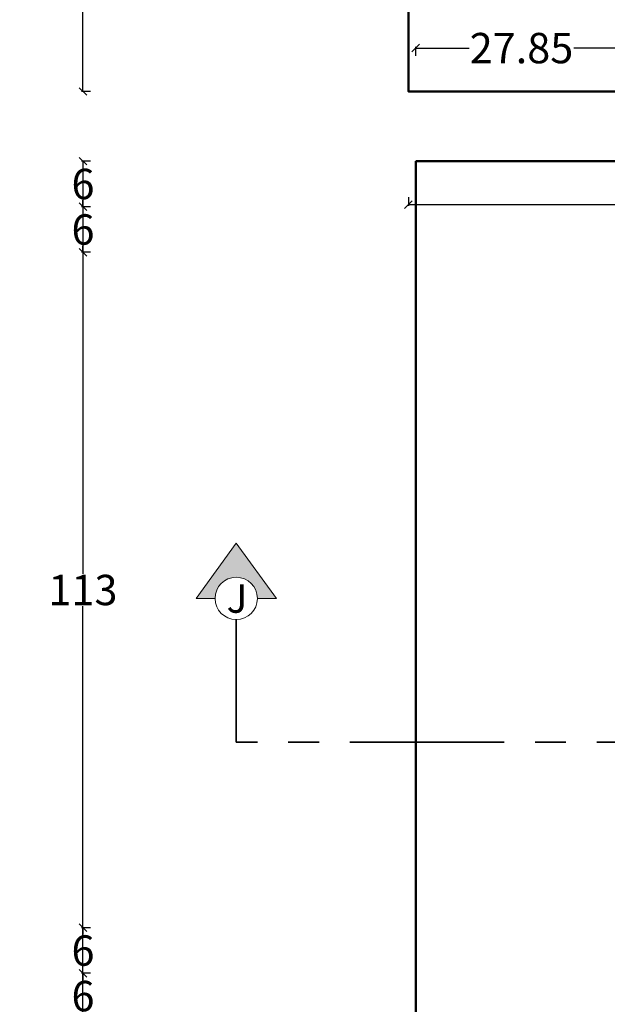
# Model space of a CAD drawing. Units: inches. Extents: x -60 to 284, y -245 to 257.
# Tile 6 of 10: x -52 to 25, y 12 to 141. Entities that reach past the tile are written whole.
import ezdxf

# ---------------------------------------------------------------- set-up
doc = ezdxf.new("R2010")
doc.units = ezdxf.units.IN
doc.header["$LTSCALE"] = 0.8
doc.header["$MEASUREMENT"] = 0
doc.linetypes.add('PHANTOM', pattern=[63.5, 31.75, -6.35, 6.35, -6.35, 6.35, -6.35])
for name, color, linetype, lineweight in [('A-ANNO-DIMS', 2, 'Continuous', 18), ('A-ANNO-SECT', 1, 'PHANTOM', 35), ('A-ANNO-SYMB', 3, 'Continuous', 18), ('A-ANNO-TEXT', 3, 'Continuous', 18), ('A-ANNO-TTLB', 7, 'Continuous', 50)]:
    doc.layers.add(name, color=color, linetype=linetype, lineweight=lineweight)
doc.styles.get("Standard").update_dxf_attribs({"font": 'arial.ttf'})
doc.dimstyles.get("Standard").update_dxf_attribs({"dimtxt": 4, "dimasz": 1, "dimexe": 0.18, "dimexo": 0.0625, "dimgap": 0.09, "dimtad": 0, "dimtih": 1, "dimtoh": 1, "dimzin": 0, "dimdsep": 46, "dimlunit": 4, "dimtxsty": 'Standard', "dimblk": 'OBLIQUE', "dimcen": 0.09, "dimadec": 0, "dimazin": 0, "dimtfac": 1, "dimtofl": 0, "dimtmove": 0, "dimatfit": 3, "dimfxl": 1, "dimfxlon": 1, "dimtolj": 1, "dimtzin": 0, "dimarcsym": 0})

# ---------------------------------------------------------------- blocks, each defined once
blk = doc.blocks.new('SECTION-MARK')
at = {"ltscale": 0.8}
for p, q in [((0, 2.79), (5.28, 10.08)), ((10.57, 2.79), (5.28, 10.08)), ((2.5, 2.79), (0, 2.79)), ((8.07, 2.79), (10.57, 2.79))]:
    blk.add_line(p, q, dxfattribs=at)
blk.add_circle((5.28, 2.79), 2.79, dxfattribs=at)
blk = doc.blocks.new('_Oblique')
at = {"color": 0, "linetype": 'ByBlock', "lineweight": -2}
blk.add_line((-0.5, -0.5), (0.5, 0.5), dxfattribs=at)
blk = doc.blocks.new('*D76')
at = {"layer": 'A-ANNO-DIMS', "color": 0, "lineweight": -2, "ltscale": 0.8, "transparency": 16777216}
for p, q in [((-0.88, 117.95), (-0.88, 116.77)), ((-0.88, 116.95), (107.9, 116.95)), ((230.43, 116.95), (121.65, 116.95)), ((230.43, 117.95), (230.43, 116.77))]:
    blk.add_line(p, q, dxfattribs=at)
at = {"layer": 'Defpoints', "color": 0, "ltscale": 0.8, "transparency": 16777216}
for p in [(-0.88, 131.85), (230.43, 131.85), (230.43, 116.95)]:
    blk.add_point(p, dxfattribs=at)
at = {"layer": 'A-ANNO-DIMS', "color": 0, "lineweight": -2, "ltscale": 0.8, "transparency": 16777216, "rotation": 180}
blk.add_blockref('_Oblique', (-0.88, 116.95), dxfattribs=at)
at = {"layer": 'A-ANNO-DIMS', "color": 0, "lineweight": -2, "ltscale": 0.8, "transparency": 16777216}
blk.add_blockref('_Oblique', (230.43, 116.95), dxfattribs=at)
at = {"layer": 'A-ANNO-DIMS', "color": 0, "ltscale": 0.8, "transparency": 16777216, "insert": (114.78, 116.95), "char_height": 4, "attachment_point": 5}
blk.add_mtext('\\A1;231.3', dxfattribs=at)
blk = doc.blocks.new('*D77')
at = {"layer": 'A-ANNO-DIMS', "color": 0, "lineweight": -2, "ltscale": 0.8, "transparency": 16777216}
for p, q in [((-42.73, 239.52), (-43.91, 239.52)), ((-43.73, 239.52), (-43.73, 187.82)), ((-43.73, 131.85), (-43.73, 183.55)), ((-42.73, 131.85), (-43.91, 131.85))]:
    blk.add_line(p, q, dxfattribs=at)
at = {"layer": 'Defpoints', "color": 0, "ltscale": 0.8, "transparency": 16777216}
for p in [(-43.73, 239.52), (-0.88, 239.52), (-0.88, 131.85)]:
    blk.add_point(p, dxfattribs=at)
at = {"layer": 'A-ANNO-DIMS', "color": 0, "lineweight": -2, "ltscale": 0.8, "transparency": 16777216}
for p, rotation in [((-43.73, 239.52), 90), ((-43.73, 131.85), 270)]:
    blk.add_blockref('_Oblique', p, dxfattribs=dict(at, rotation=rotation))
at = {"layer": 'A-ANNO-DIMS', "color": 0, "ltscale": 0.8, "transparency": 16777216, "insert": (-43.73, 185.69), "char_height": 4, "attachment_point": 5}
blk.add_mtext('\\A1;107.66', dxfattribs=at)
blk = doc.blocks.new('*D90')
at = {"layer": 'A-ANNO-DIMS', "color": 0, "lineweight": -2, "ltscale": 0.8, "transparency": 16777216}
for p, q in [((-42.73, 122.67), (-43.91, 122.67)), ((-43.73, 122.67), (-43.73, 68.3)), ((-43.73, 9.67), (-43.73, 64.03)), ((-42.73, 9.67), (-43.91, 9.67))]:
    blk.add_line(p, q, dxfattribs=at)
at = {"layer": 'Defpoints', "color": 0, "ltscale": 0.8, "transparency": 16777216}
for p in [(-43.73, 122.67), (0.09, 122.67), (0.09, 9.67)]:
    blk.add_point(p, dxfattribs=at)
at = {"layer": 'A-ANNO-DIMS', "color": 0, "lineweight": -2, "ltscale": 0.8, "transparency": 16777216}
for p, rotation in [((-43.73, 122.67), 90), ((-43.73, 9.67), 270)]:
    blk.add_blockref('_Oblique', p, dxfattribs=dict(at, rotation=rotation))
at = {"layer": 'A-ANNO-DIMS', "color": 0, "ltscale": 0.8, "transparency": 16777216, "insert": (-43.73, 66.17), "char_height": 4, "attachment_point": 5}
blk.add_mtext('\\A1;113', dxfattribs=at)
blk = doc.blocks.new('*D91')
at = {"layer": 'A-ANNO-DIMS', "color": 0, "lineweight": -2, "ltscale": 0.8, "transparency": 16777216}
for p, q in [((0.09, 136.57), (0.09, 137.75)), ((0.09, 137.57), (7.12, 137.57)), ((27.94, 137.57), (20.9, 137.57)), ((27.94, 136.57), (27.94, 137.75))]:
    blk.add_line(p, q, dxfattribs=at)
at = {"layer": 'Defpoints', "color": 0, "ltscale": 0.8, "transparency": 16777216}
for p in [(27.94, 137.57), (0.09, 122.67), (27.94, 122.67)]:
    blk.add_point(p, dxfattribs=at)
at = {"layer": 'A-ANNO-DIMS', "color": 0, "lineweight": -2, "ltscale": 0.8, "transparency": 16777216, "rotation": 180}
blk.add_blockref('_Oblique', (0.09, 137.57), dxfattribs=at)
at = {"layer": 'A-ANNO-DIMS', "color": 0, "lineweight": -2, "ltscale": 0.8, "transparency": 16777216}
blk.add_blockref('_Oblique', (27.94, 137.57), dxfattribs=at)
at = {"layer": 'A-ANNO-DIMS', "color": 0, "ltscale": 0.8, "transparency": 16777216, "insert": (14.01, 137.57), "char_height": 4, "attachment_point": 5}
blk.add_mtext('\\A1;27.85', dxfattribs=at)
blk = doc.blocks.new('*D99')
at = {"layer": 'A-ANNO-DIMS', "color": 0, "lineweight": -2, "ltscale": 0.8, "transparency": 16777216}
for p, q in [((-42.73, 122.67), (-43.91, 122.67)), ((-43.73, 122.67), (-43.73, 121.8)), ((-43.73, 116.67), (-43.73, 117.53)), ((-42.73, 116.67), (-43.91, 116.67))]:
    blk.add_line(p, q, dxfattribs=at)
at = {"layer": 'Defpoints', "color": 0, "ltscale": 0.8, "transparency": 16777216}
for p in [(-43.73, 122.67), (33.94, 122.67), (33.94, 116.67)]:
    blk.add_point(p, dxfattribs=at)
at = {"layer": 'A-ANNO-DIMS', "color": 0, "lineweight": -2, "ltscale": 0.8, "transparency": 16777216}
for p, rotation in [((-43.73, 122.67), 90), ((-43.73, 116.67), 270)]:
    blk.add_blockref('_Oblique', p, dxfattribs=dict(at, rotation=rotation))
at = {"layer": 'A-ANNO-DIMS', "color": 0, "ltscale": 0.8, "transparency": 16777216, "insert": (-43.73, 119.67), "char_height": 4, "attachment_point": 5}
blk.add_mtext('\\A1;6', dxfattribs=at)
blk = doc.blocks.new('*D100')
at = {"layer": 'A-ANNO-DIMS', "color": 0, "lineweight": -2, "ltscale": 0.8, "transparency": 16777216}
for p, q in [((-42.73, 116.67), (-43.91, 116.67)), ((-43.73, 116.67), (-43.73, 115.8)), ((-42.73, 110.67), (-43.91, 110.67)), ((-43.73, 110.67), (-43.73, 111.53))]:
    blk.add_line(p, q, dxfattribs=at)
at = {"layer": 'Defpoints', "color": 0, "ltscale": 0.8, "transparency": 16777216}
for p in [(-43.73, 116.67), (33.94, 116.67), (32.94, 110.67)]:
    blk.add_point(p, dxfattribs=at)
at = {"layer": 'A-ANNO-DIMS', "color": 0, "lineweight": -2, "ltscale": 0.8, "transparency": 16777216}
for p, rotation in [((-43.73, 116.67), 90), ((-43.73, 110.67), 270)]:
    blk.add_blockref('_Oblique', p, dxfattribs=dict(at, rotation=rotation))
at = {"layer": 'A-ANNO-DIMS', "color": 0, "ltscale": 0.8, "transparency": 16777216, "insert": (-43.73, 113.67), "char_height": 4, "attachment_point": 5}
blk.add_mtext('\\A1;6', dxfattribs=at)
blk = doc.blocks.new('*D101')
at = {"layer": 'A-ANNO-DIMS', "color": 0, "lineweight": -2, "ltscale": 0.8, "transparency": 16777216}
for p, q in [((-42.73, 15.67), (-43.91, 15.67)), ((-43.73, 15.67), (-43.73, 14.8)), ((-43.73, 9.67), (-43.73, 10.53)), ((-42.73, 9.67), (-43.91, 9.67))]:
    blk.add_line(p, q, dxfattribs=at)
at = {"layer": 'Defpoints', "color": 0, "ltscale": 0.8, "transparency": 16777216}
for p in [(-43.73, 15.67), (33.94, 15.67), (33.94, 9.67)]:
    blk.add_point(p, dxfattribs=at)
at = {"layer": 'A-ANNO-DIMS', "color": 0, "lineweight": -2, "ltscale": 0.8, "transparency": 16777216}
for p, rotation in [((-43.73, 15.67), 90), ((-43.73, 9.67), 270)]:
    blk.add_blockref('_Oblique', p, dxfattribs=dict(at, rotation=rotation))
at = {"layer": 'A-ANNO-DIMS', "color": 0, "ltscale": 0.8, "transparency": 16777216, "insert": (-43.73, 12.67), "char_height": 4, "attachment_point": 5}
blk.add_mtext('\\A1;6', dxfattribs=at)
blk = doc.blocks.new('*D102')
at = {"layer": 'A-ANNO-DIMS', "color": 0, "lineweight": -2, "ltscale": 0.8, "transparency": 16777216}
for p, q in [((-42.73, 21.67), (-43.91, 21.67)), ((-43.73, 21.67), (-43.73, 20.8)), ((-42.73, 15.67), (-43.91, 15.67)), ((-43.73, 15.67), (-43.73, 16.53))]:
    blk.add_line(p, q, dxfattribs=at)
at = {"layer": 'Defpoints', "color": 0, "ltscale": 0.8, "transparency": 16777216}
for p in [(32.94, 21.67), (-43.73, 15.67), (33.94, 15.67)]:
    blk.add_point(p, dxfattribs=at)
at = {"layer": 'A-ANNO-DIMS', "color": 0, "lineweight": -2, "ltscale": 0.8, "transparency": 16777216}
for p, rotation in [((-43.73, 21.67), 90), ((-43.73, 15.67), 270)]:
    blk.add_blockref('_Oblique', p, dxfattribs=dict(at, rotation=rotation))
at = {"layer": 'A-ANNO-DIMS', "color": 0, "ltscale": 0.8, "transparency": 16777216, "insert": (-43.73, 18.67), "char_height": 4, "attachment_point": 5}
blk.add_mtext('\\A1;6', dxfattribs=at)

msp = doc.modelspace()

# ---------------------------------------------------------------- hatches: boundary and pattern name
at = {"layer": 'A-ANNO-SYMB', "ltscale": 0.8}
h = msp.add_hatch(color=256, dxfattribs=at)
h.dxf.hatch_style = 1
h.paths.add_polyline_path([(-23.5489, 72.3512), (-28.8318, 65.0558), (-26.3347, 65.0558, -1), (-20.7631, 65.0558), (-18.2661, 65.0558)])

# ---------------------------------------------------------------- linework, layer by layer
at = {"layer": 'A-ANNO-SECT', "ltscale": 0.8}
for p in [(-23.5489, 62.27), (255.5807, 46.116)]:
    msp.add_line(p, (-23.5489, 46.116), dxfattribs=at)
at = {"layer": 'A-ANNO-TTLB', "ltscale": 0.8}
for points in [[(-0.8787, 239.5184), (230.4297, 239.5184), (230.4297, 131.8542), (-0.8787, 131.8542)], [(0.0867, 122.666), (239.6639, 122.666), (239.6639, 9.666), (0.0867, 9.666)]]:
    msp.add_lwpolyline(points, close=True, dxfattribs=at)

# ---------------------------------------------------------------- block references
at = {"layer": 'A-ANNO-SYMB'}
msp.add_blockref('SECTION-MARK', (-28.8316, 62.27), dxfattribs=at)

# ---------------------------------------------------------------- texts
at = {"layer": 'A-ANNO-TEXT', "ltscale": 0.8, "insert": (-24.8197, 66.9248), "char_height": 3.7545, "attachment_point": 1}
msp.add_mtext_dynamic_manual_height_columns('J', width=2.355391, gutter_width=0.4172, heights=[0], dxfattribs=at)

# ---------------------------------------------------------------- dimensions: what is measured, and where the dimension line sits
at = {"layer": 'A-ANNO-DIMS', "ltscale": 0.8}
for base, p1, p2, override, picture, middle in [((-43.7318, 239.5184), (-0.8787, 131.8542), (-0.8787, 239.5184), {"dimdec": 2, "dimlfac": 1, "dimrnd": 0, "dimzin": 0, "dimdsep": 46, "dimlunit": 2}, '*D77', (-43.7318, 185.6863)), ((-43.7318, 122.666), (0.0867, 9.666), (0.0867, 122.666), {"dimdec": 0, "dimlfac": 1, "dimrnd": 0, "dimzin": 0, "dimdsep": 46, "dimlunit": 2}, '*D90', (-43.7318, 66.166)), ((-43.7318, 122.666), (33.9361, 116.666), (33.9361, 122.666), {"dimdec": 0, "dimlfac": 1, "dimrnd": 0, "dimzin": 0, "dimdsep": 46, "dimlunit": 2}, '*D99', (-43.7318, 119.666)), ((-43.7318, 116.666), (32.9361, 110.666), (33.9361, 116.666), {"dimdec": 0, "dimlfac": 1, "dimrnd": 0, "dimzin": 0, "dimdsep": 46, "dimlunit": 2}, '*D100', (-43.7318, 113.666)), ((-43.7318, 15.666), (32.9361, 21.666), (33.9361, 15.666), {"dimdec": 0, "dimlfac": 1, "dimrnd": 0, "dimzin": 0, "dimdsep": 46, "dimlunit": 2}, '*D102', (-43.7318, 18.666)), ((-43.7318, 15.666), (33.9361, 9.666), (33.9361, 15.666), {"dimdec": 0, "dimlfac": 1, "dimrnd": 0, "dimzin": 0, "dimdsep": 46, "dimlunit": 2}, '*D101', (-43.7318, 12.666))]:
    dim = msp.add_linear_dim(base=base, p1=p1, p2=p2, angle=90, dimstyle='Standard', override=override, dxfattribs=at)
    dim.commit()
    dim.dimension.update_dxf_attribs({"geometry": picture, "text_midpoint": middle})
for base, p1, p2, override, picture, middle in [((27.9361, 137.566), (0.0867, 122.666), (27.9361, 122.666), {"dimdec": 2, "dimlfac": 1, "dimrnd": 0, "dimzin": 0, "dimdsep": 46, "dimlunit": 2}, '*D91', (14.0114, 137.566)), ((230.4297, 116.9542), (-0.8787, 131.8542), (230.4297, 131.8542), {"dimdec": 1, "dimlfac": 1, "dimrnd": 0, "dimzin": 0, "dimdsep": 46, "dimlunit": 2}, '*D76', (114.7755, 116.9542))]:
    dim = msp.add_linear_dim(base=base, p1=p1, p2=p2, dimstyle='Standard', override=override, dxfattribs=at)
    dim.commit()
    dim.dimension.update_dxf_attribs({"geometry": picture, "text_midpoint": middle})

doc.saveas('drawing.dxf')
